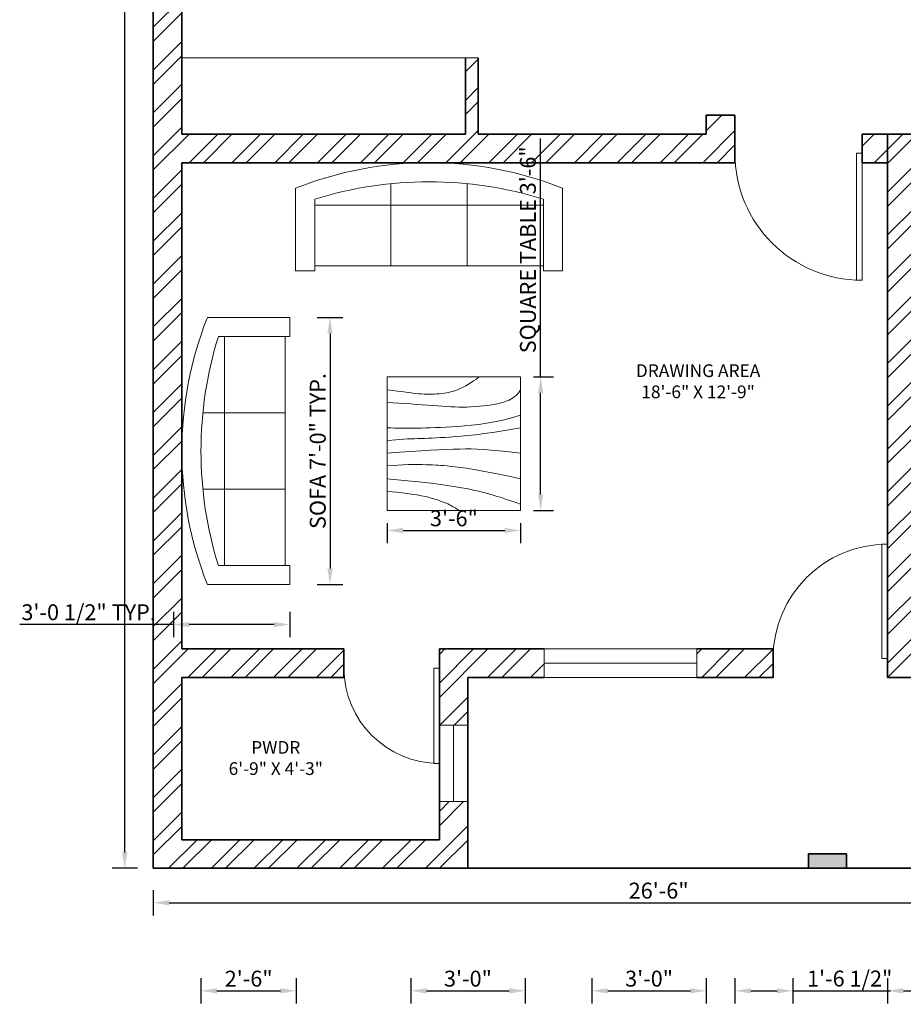
# Model space of a CAD drawing. Units: inches. Extents: x 468 to 1096, y 138 to 946.
# Tile 1 of 6: x 471 to 749, y 138 to 448. Entities that reach past the tile are written whole.
import ezdxf

# ---------------------------------------------------------------- set-up
doc = ezdxf.new("R2010")
doc.units = ezdxf.units.IN
for name, color, linetype, lineweight in [('A-ANNO-DIMS', 2, 'Continuous', 18), ('A-AREA-IDEN', 7, 'Continuous', 18), ('A-DOOR', 3, 'Continuous', 18), ('A-FLOR-CASE', 9, 'Continuous', 18), ('A-FURN', 8, 'Continuous', 18), ('A-GLAZ', 4, 'Continuous', 18), ('A-SITE-GATE', 7, 'Continuous', 35), ('A-SITE-PATT', 8, 'Continuous', 13), ('A-WALL', 7, 'Continuous', 35), ('A-WALL-PATT', 8, 'Continuous', 13), ('C-PROP', 7, 'Continuous', 35)]:
    doc.layers.add(name, color=color, linetype=linetype, lineweight=lineweight)
doc.styles.get("Standard").update_dxf_attribs({"font": 'arial.ttf'})
doc.dimstyles.new('ISO-25', dxfattribs={"dimtxt": 5, "dimasz": 5, "dimexe": 4, "dimexo": 4, "dimtad": 1, "dimdec": 1, "dimlunit": 3, "dimtxsty": 'Standard', "dimcen": 2.5, "dimadec": 0, "dimazin": 0, "dimtfac": 1, "dimtdec": 1, "dimtmove": 0, "dimatfit": 3, "dimfxl": 4, "dimfxlon": 1, "dimarcsym": 0})

# ---------------------------------------------------------------- blocks, each defined once
blk = doc.blocks.new('*U7')
for p, q in [((-40, 0), (-40, 6)), ((0, 0), (0, 6))]:
    blk.add_line(p, q)
blk.add_lwpolyline([(0, 0), (0, -40), (-1.75, -40), (-1.75, 0)], close=True)
blk.add_arc((0, 0), 40, 180, 270)
blk = doc.blocks.new('*U3')
for p, q in [((0, 0), (0, -6)), ((-36, 0), (-36, -6))]:
    blk.add_line(p, q)
blk.add_lwpolyline([(0, 0), (0, 36), (-1.75, 36), (-1.75, 0)], close=True)
blk.add_arc((0, 0), 36, 90, 180)
blk = doc.blocks.new('*U8')
for p, q in [((-30, 0), (-30, 6)), ((0, 0), (0, 6))]:
    blk.add_line(p, q)
blk.add_lwpolyline([(0, 0), (0, -30), (-1.75, -30), (-1.75, 0)], close=True)
blk.add_arc((0, 0), 30, 180, 270)
blk = doc.blocks.new('Table - Square Woodgrain 42 x 42 in.')
blk.add_line((0, -42), (42, -42))
for points in [[(0, -4), (1.704, -4.2172), (3.2358, -4.4188), (4.615, -4.604), (5.8615, -4.7721), (6.9951, -4.9224), (8.0357, -5.0541), (9.0031, -5.1667), (9.9171, -5.2594), (10.7951, -5.3316), (11.6445, -5.3836), (12.4702, -5.4157), (13.277, -5.4283), (14.0698, -5.4217), (14.8535, -5.3964), (15.6331, -5.3526), (16.4133, -5.2908), (17.1986, -5.2103), (17.9913, -5.1062), (18.793, -4.9727), (19.6056, -4.8038), (20.4307, -4.5937), (21.2701, -4.3365), (22.1256, -4.0262), (22.9989, -3.6571), (23.888, -3.2272), (24.7756, -2.7516), (25.6408, -2.2491), (26.4624, -1.7387), (27.2195, -1.2395), (27.891, -0.7703), (28.456, -0.3501), (28.8934, 0.002)], [(0, -42), (0, 0), (42, 0), (42, -42)], [(0, -8), (1.8203, -8.1001), (3.6741, -8.2149), (5.5411, -8.3408), (7.4011, -8.4741), (9.2339, -8.6112), (11.0193, -8.7484), (12.7371, -8.8821), (14.3671, -9.0086), (15.8954, -9.1246), (17.3337, -9.2278), (18.6997, -9.3159), (20.0116, -9.387), (21.2871, -9.4389), (22.5442, -9.4696), (23.8008, -9.477), (25.0749, -9.459), (26.3791, -9.4137), (27.7049, -9.3403), (29.0383, -9.2382), (30.3655, -9.1068), (31.6728, -8.9455), (32.9461, -8.7535), (34.1717, -8.5304), (35.3358, -8.2756), (36.4268, -7.9863), (37.443, -7.6521), (38.3849, -7.2603), (39.253, -6.7986), (40.048, -6.2542), (40.7705, -5.6147), (41.421, -4.8674), (42, -4)], [(42, -12), (39.1784, -12.8621), (36.4519, -13.5654), (33.8246, -14.1294), (31.3004, -14.5731), (28.8832, -14.9161), (26.577, -15.1775), (24.3858, -15.3768), (22.3136, -15.5332), (20.3622, -15.6632), (18.5254, -15.7718), (16.7947, -15.8612), (15.1618, -15.9338), (13.6183, -15.9916), (12.1558, -16.0369), (10.7659, -16.0718), (9.4403, -16.0987), (8.1703, -16.1191), (6.9461, -16.1325), (5.7577, -16.1377), (4.595, -16.1335), (3.4479, -16.1188), (2.3064, -16.0924), (1.1604, -16.0532), (0, -16)], [(42, -16), (37.6529, -16.7365), (33.8802, -17.329), (30.6179, -17.7961), (27.8015, -18.1561), (25.3668, -18.4275), (23.2497, -18.6288), (21.3859, -18.7785), (19.7111, -18.8949), (18.1693, -18.9939), (16.7375, -19.0795), (15.401, -19.1534), (14.1449, -19.217), (12.9544, -19.2717), (11.8148, -19.3191), (10.7113, -19.3606), (9.6291, -19.3976), (8.5534, -19.4323), (7.47, -19.4689), (6.3643, -19.5122), (5.222, -19.5672), (4.0288, -19.6386), (2.7703, -19.7313), (1.4321, -19.8501), (0, -20)], [(0, -24), (3.9243, -23.6805), (7.4766, -23.4138), (10.6891, -23.1954), (13.5943, -23.0205), (16.2247, -22.8847), (18.6125, -22.7832), (20.7903, -22.7116), (22.7903, -22.6651), (24.6563, -22.642), (26.4764, -22.6507), (28.35, -22.7024), (30.3766, -22.8084), (32.6555, -22.98), (35.2861, -23.2283), (38.3678, -23.5645), (42, -24)], [(42, -32), (37.392, -31.017), (33.4585, -30.2231), (30.1291, -29.5949), (27.3334, -29.109), (25.0009, -28.742), (23.0612, -28.4707), (21.4439, -28.2716), (20.0786, -28.1215), (18.8998, -28.0002), (17.8609, -27.9014), (16.9206, -27.8219), (16.0371, -27.7588), (15.1691, -27.709), (14.2748, -27.6693), (13.3128, -27.6368), (12.2415, -27.6083), (11.0295, -27.5824), (9.6867, -27.5643), (8.233, -27.5608), (6.6884, -27.5787), (5.0728, -27.6248), (3.4062, -27.7058), (1.7086, -27.8286), (0, -28)], [(0, -32), (5.4026, -32.5358), (9.9494, -33.019), (13.7424, -33.4553), (16.8834, -33.8505), (19.4743, -34.2106), (21.6171, -34.5413), (23.4136, -34.8486), (24.9657, -35.1382), (26.3614, -35.4156), (27.6332, -35.6841), (28.7995, -35.9467), (29.8788, -36.2064), (30.8897, -36.4661), (31.8507, -36.7288), (32.7802, -36.9973), (33.6968, -37.2747), (34.6175, -37.5635), (35.5531, -37.8651), (36.5128, -38.1805), (37.506, -38.5108), (38.5421, -38.8568), (39.6302, -39.2197), (40.7797, -39.6004), (42, -40)], [(0, -36), (3.0098, -36.2857), (5.5354, -36.5643), (7.6368, -36.8359), (9.374, -37.1009), (10.807, -37.3597), (11.9957, -37.6126), (13.0002, -37.8599), (13.8804, -38.102), (14.6874, -38.3393), (15.4365, -38.5729), (16.1338, -38.8041), (16.7858, -39.0341), (17.3987, -39.264), (17.9787, -39.4952), (18.5322, -39.7288), (19.0655, -39.9662), (19.5832, -40.2081), (20.0842, -40.4544), (20.5657, -40.7046), (21.0249, -40.9581), (21.459, -41.2144), (21.8653, -41.4731), (22.2409, -41.7335), (22.5831, -41.9951)]]:
    blk.add_lwpolyline(points)
blk = doc.blocks.new('Sofa - Roundback 7 ft.')
for p, q in [((-12.00002, -32.4421), (-12.00003, -6.5971)), ((11.99997, -32.4421), (11.99998, -6.5971)), ((-36.000027, -34), (-36.000027, -11.4696)), ((35.99998, -34), (35.99998, -11.4696)), ((-35.999844, -13.3819), (35.9998, -13.3819)), ((-36.000027, -32.4421), (35.99998, -32.4421))]:
    blk.add_line(p, q)
for points in [[(-36.000027, -34), (-42.000027, -34), (-42.000027, -8)], [(41.99998, -8), (41.99998, -34), (35.99998, -34)]]:
    blk.add_lwpolyline(points)
for centre, radius, start, end in [((0, -114.25), 114.25, 68.43141, 111.5686), ((-0.00001, -127.1968), 121.1968, 72.72033, 107.2797)]:
    blk.add_arc(centre, radius, start, end)
blk = doc.blocks.new('*D18')
at = {"layer": 'A-ANNO-DIMS', "color": 0, "lineweight": -2, "transparency": 16777216}
for p, q in [((508.14, 901.16), (500.14, 901.16)), ((504.14, 186.16), (504.14, 896.16)), ((508.14, 181.16), (500.14, 181.16))]:
    blk.add_line(p, q, dxfattribs=at)
at = {"layer": 'A-ANNO-DIMS', "color": 0, "transparency": 16777216}
for points in [[(503.3, 896.16), (504.97, 896.16), (504.14, 901.16)], [(503.3, 186.16), (504.97, 186.16), (504.14, 181.16)]]:
    blk.add_solid(points, dxfattribs=at)
at = {"layer": 'Defpoints', "color": 0, "transparency": 16777216}
for p in [(504.14, 901.16), (513.13, 901.16), (513.13, 181.16)]:
    blk.add_point(p, dxfattribs=at)
at = {"layer": 'A-ANNO-DIMS', "color": 0, "transparency": 16777216, "insert": (500.96, 541.16), "char_height": 5, "attachment_point": 5, "rotation": 90}
blk.add_mtext("60'", dxfattribs=at)
blk = doc.blocks.new('*D19')
at = {"layer": 'A-ANNO-DIMS', "color": 0, "lineweight": -2, "transparency": 16777216}
for p, q in [((513.13, 174.32), (513.13, 166.32)), ((831.13, 174.32), (831.13, 166.32)), ((518.13, 170.32), (826.13, 170.32))]:
    blk.add_line(p, q, dxfattribs=at)
at = {"layer": 'A-ANNO-DIMS', "color": 0, "transparency": 16777216}
for points in [[(518.13, 171.15), (518.13, 169.48), (513.13, 170.32)], [(826.13, 171.15), (826.13, 169.48), (831.13, 170.32)]]:
    blk.add_solid(points, dxfattribs=at)
at = {"layer": 'Defpoints', "color": 0, "transparency": 16777216}
for p in [(513.13, 181.16), (831.13, 181.16), (831.13, 170.32)]:
    blk.add_point(p, dxfattribs=at)
at = {"layer": 'A-ANNO-DIMS', "color": 0, "transparency": 16777216, "insert": (672.13, 173.49), "char_height": 5, "attachment_point": 5}
blk.add_mtext('26\'-6"', dxfattribs=at)
blk = doc.blocks.new('WIN-24-W9')
for p, q in [((0, 24), (9, 24)), ((4.5, 24), (4.5, 0)), ((0, 0), (9, 0))]:
    blk.add_line(p, q)
blk = doc.blocks.new('WIN-48-W9')
for p, q in [((0, 0), (0, 9)), ((48, 0), (48, 9)), ((0, 4.5), (48, 4.5))]:
    blk.add_line(p, q)
blk = doc.blocks.new('*D37')
at = {"layer": 'A-ANNO-DIMS', "color": 0, "lineweight": -2, "transparency": 16777216}
for p, q in [((564.73, 354.45), (572.73, 354.45)), ((568.73, 349.45), (568.73, 275.45)), ((564.73, 270.45), (572.73, 270.45))]:
    blk.add_line(p, q, dxfattribs=at)
at = {"layer": 'A-ANNO-DIMS', "color": 0, "transparency": 16777216}
for points in [[(567.9, 349.45), (569.56, 349.45), (568.73, 354.45)], [(567.9, 275.45), (569.56, 275.45), (568.73, 270.45)]]:
    blk.add_solid(points, dxfattribs=at)
at = {"layer": 'Defpoints', "color": 0, "transparency": 16777216}
for p in [(556.13, 354.45), (556.13, 270.45), (568.73, 270.45)]:
    blk.add_point(p, dxfattribs=at)
at = {"layer": 'A-ANNO-DIMS', "color": 0, "transparency": 16777216, "insert": (565.52, 312.45), "char_height": 5, "attachment_point": 5, "rotation": 90}
blk.add_mtext('SOFA 7\'-0" TYP.', dxfattribs=at)
blk = doc.blocks.new('*D38')
at = {"layer": 'A-ANNO-DIMS', "color": 0, "lineweight": -2, "transparency": 16777216}
for p, q in [((519.46, 261.85), (519.46, 253.85)), ((556.13, 261.85), (556.13, 253.85)), ((519.46, 257.85), (471.09, 257.85)), ((551.13, 257.85), (524.46, 257.85))]:
    blk.add_line(p, q, dxfattribs=at)
at = {"layer": 'A-ANNO-DIMS', "color": 0, "transparency": 16777216}
for points in [[(524.46, 258.69), (524.46, 257.02), (519.46, 257.85)], [(551.13, 258.69), (551.13, 257.02), (556.13, 257.85)]]:
    blk.add_solid(points, dxfattribs=at)
at = {"layer": 'Defpoints', "color": 0, "transparency": 16777216}
for p in [(519.46, 270.45), (556.13, 270.45), (519.46, 257.85)]:
    blk.add_point(p, dxfattribs=at)
at = {"layer": 'A-ANNO-DIMS', "color": 0, "transparency": 16777216, "insert": (492.78, 261.07), "char_height": 5, "attachment_point": 5}
blk.add_mtext('3\'-0 1/2" TYP.', dxfattribs=at)
blk = doc.blocks.new('*D53')
at = {"layer": 'A-ANNO-DIMS', "color": 0, "lineweight": -2, "transparency": 16777216}
for p, q in [((635.01, 335.75), (635.01, 410.78)), ((632.71, 335.75), (639.01, 335.75)), ((635.01, 298.75), (635.01, 330.75)), ((632.71, 293.75), (639.01, 293.75))]:
    blk.add_line(p, q, dxfattribs=at)
at = {"layer": 'A-ANNO-DIMS', "color": 0, "transparency": 16777216}
for points in [[(634.18, 330.75), (635.84, 330.75), (635.01, 335.75)], [(634.18, 298.75), (635.84, 298.75), (635.01, 293.75)]]:
    blk.add_solid(points, dxfattribs=at)
at = {"layer": 'Defpoints', "color": 0, "transparency": 16777216}
for p in [(628.71, 335.75), (635.01, 335.75), (628.71, 293.75)]:
    blk.add_point(p, dxfattribs=at)
at = {"layer": 'A-ANNO-DIMS', "color": 0, "transparency": 16777216, "insert": (631.65, 375.76), "char_height": 5, "attachment_point": 5, "rotation": 90}
blk.add_mtext('SQUARE TABLE 3\'-6"', dxfattribs=at)
blk = doc.blocks.new('*D54')
at = {"layer": 'A-ANNO-DIMS', "color": 0, "lineweight": -2, "transparency": 16777216}
for p, q in [((586.71, 289.75), (586.71, 283.45)), ((628.71, 289.75), (628.71, 283.45)), ((591.71, 287.45), (623.71, 287.45))]:
    blk.add_line(p, q, dxfattribs=at)
at = {"layer": 'A-ANNO-DIMS', "color": 0, "transparency": 16777216}
for points in [[(591.71, 288.28), (591.71, 286.62), (586.71, 287.45)], [(623.71, 288.28), (623.71, 286.62), (628.71, 287.45)]]:
    blk.add_solid(points, dxfattribs=at)
at = {"layer": 'Defpoints', "color": 0, "transparency": 16777216}
for p in [(586.71, 293.75), (628.71, 293.75), (628.71, 287.45)]:
    blk.add_point(p, dxfattribs=at)
at = {"layer": 'A-ANNO-DIMS', "color": 0, "transparency": 16777216, "insert": (607.71, 290.63), "char_height": 5, "attachment_point": 5}
blk.add_mtext('3\'-6"', dxfattribs=at)
blk = doc.blocks.new('*D55')
at = {"layer": 'A-ANNO-DIMS', "color": 0, "lineweight": -2, "transparency": 16777216}
for p, q in [((744.13, 146.61), (744.13, 138.61)), ((858.13, 146.61), (858.13, 138.61)), ((749.13, 142.61), (853.13, 142.61))]:
    blk.add_line(p, q, dxfattribs=at)
at = {"layer": 'A-ANNO-DIMS', "color": 0, "transparency": 16777216}
for points in [[(749.13, 143.44), (749.13, 141.78), (744.13, 142.61)], [(853.13, 143.44), (853.13, 141.78), (858.13, 142.61)]]:
    blk.add_solid(points, dxfattribs=at)
at = {"layer": 'Defpoints', "color": 0, "transparency": 16777216}
for p in [(744.13, 241.16), (858.13, 241.16), (858.13, 142.61)]:
    blk.add_point(p, dxfattribs=at)
at = {"layer": 'A-ANNO-DIMS', "color": 0, "transparency": 16777216, "insert": (801.13, 145.79), "char_height": 5, "attachment_point": 5}
blk.add_mtext('9\'-6"', dxfattribs=at)
blk = doc.blocks.new('*D61')
at = {"layer": 'A-ANNO-DIMS', "color": 0, "lineweight": -2, "transparency": 16777216}
for p, q in [((594.13, 146.61), (594.13, 138.61)), ((630.13, 146.61), (630.13, 138.61)), ((599.13, 142.61), (625.13, 142.61))]:
    blk.add_line(p, q, dxfattribs=at)
at = {"layer": 'A-ANNO-DIMS', "color": 0, "transparency": 16777216}
for points in [[(599.13, 143.44), (599.13, 141.78), (594.13, 142.61)], [(625.13, 143.44), (625.13, 141.78), (630.13, 142.61)]]:
    blk.add_solid(points, dxfattribs=at)
at = {"layer": 'Defpoints', "color": 0, "transparency": 16777216}
for p in [(594.13, 829.16), (630.13, 826.16), (630.13, 142.61)]:
    blk.add_point(p, dxfattribs=at)
at = {"layer": 'A-ANNO-DIMS', "color": 0, "transparency": 16777216, "insert": (612.13, 145.79), "char_height": 5, "attachment_point": 5}
blk.add_mtext('3\'-0"', dxfattribs=at)
blk = doc.blocks.new('*D66')
at = {"layer": 'A-ANNO-DIMS', "color": 0, "lineweight": -2, "transparency": 16777216}
for p, q in [((696.13, 146.61), (696.13, 138.61)), ((714.39, 146.61), (714.39, 138.61)), ((701.13, 142.61), (709.39, 142.61)), ((714.39, 142.61), (745.11, 142.61))]:
    blk.add_line(p, q, dxfattribs=at)
at = {"layer": 'A-ANNO-DIMS', "color": 0, "transparency": 16777216}
for points in [[(701.13, 143.44), (701.13, 141.78), (696.13, 142.61)], [(709.39, 143.44), (709.39, 141.78), (714.39, 142.61)]]:
    blk.add_solid(points, dxfattribs=at)
at = {"layer": 'Defpoints', "color": 0, "transparency": 16777216}
for p in [(696.13, 820.16), (714.39, 802.16), (714.39, 142.61)]:
    blk.add_point(p, dxfattribs=at)
at = {"layer": 'A-ANNO-DIMS', "color": 0, "transparency": 16777216, "insert": (732.25, 145.82), "char_height": 5, "attachment_point": 5}
blk.add_mtext('1\'-6 1/2"', dxfattribs=at)
blk = doc.blocks.new('*D75')
at = {"layer": 'A-ANNO-DIMS', "color": 0, "lineweight": -2, "transparency": 16777216}
for p, q in [((696.13, 935.71), (696.13, 943.71)), ((736.13, 935.71), (736.13, 943.71)), ((701.13, 939.71), (731.13, 939.71))]:
    blk.add_line(p, q, dxfattribs=at)
at = {"layer": 'A-ANNO-DIMS', "color": 0, "transparency": 16777216}
for points in [[(701.13, 940.54), (701.13, 938.88), (696.13, 939.71)], [(731.13, 940.54), (731.13, 938.88), (736.13, 939.71)]]:
    blk.add_solid(points, dxfattribs=at)
at = {"layer": 'Defpoints', "color": 0, "transparency": 16777216}
for p in [(736.13, 939.71), (696.13, 412.16), (736.13, 412.16)]:
    blk.add_point(p, dxfattribs=at)
at = {"layer": 'A-ANNO-DIMS', "color": 0, "transparency": 16777216, "insert": (716.13, 942.89), "char_height": 5, "attachment_point": 5}
blk.add_mtext('3\'-4"', dxfattribs=at)
blk = doc.blocks.new('*D76')
at = {"layer": 'A-ANNO-DIMS', "color": 0, "lineweight": -2, "transparency": 16777216}
for p, q in [((1087.68, 454.16), (1095.68, 454.16)), ((1091.68, 423.16), (1091.68, 449.16)), ((1087.68, 418.16), (1095.68, 418.16))]:
    blk.add_line(p, q, dxfattribs=at)
at = {"layer": 'A-ANNO-DIMS', "color": 0, "transparency": 16777216}
for points in [[(1090.85, 449.16), (1092.51, 449.16), (1091.68, 454.16)], [(1090.85, 423.16), (1092.51, 423.16), (1091.68, 418.16)]]:
    blk.add_solid(points, dxfattribs=at)
at = {"layer": 'Defpoints', "color": 0, "transparency": 16777216}
for p in [(687.13, 454.16), (1091.68, 454.16), (687.13, 418.16)]:
    blk.add_point(p, dxfattribs=at)
at = {"layer": 'A-ANNO-DIMS', "color": 0, "transparency": 16777216, "insert": (1088.5, 436.16), "char_height": 5, "attachment_point": 5, "rotation": 90}
blk.add_mtext('3\'-0"', dxfattribs=at)
blk = doc.blocks.new('*D77')
at = {"layer": 'A-ANNO-DIMS', "color": 0, "lineweight": -2, "transparency": 16777216}
for p, q in [((651.13, 146.61), (651.13, 138.61)), ((687.13, 146.61), (687.13, 138.61)), ((656.13, 142.61), (682.13, 142.61))]:
    blk.add_line(p, q, dxfattribs=at)
at = {"layer": 'A-ANNO-DIMS', "color": 0, "transparency": 16777216}
for points in [[(656.13, 143.44), (656.13, 141.78), (651.13, 142.61)], [(682.13, 143.44), (682.13, 141.78), (687.13, 142.61)]]:
    blk.add_solid(points, dxfattribs=at)
at = {"layer": 'Defpoints', "color": 0, "transparency": 16777216}
for p in [(651.13, 565.16), (687.13, 565.16), (687.13, 142.61)]:
    blk.add_point(p, dxfattribs=at)
at = {"layer": 'A-ANNO-DIMS', "color": 0, "transparency": 16777216, "insert": (669.13, 145.79), "char_height": 5, "attachment_point": 5}
blk.add_mtext('3\'-0"', dxfattribs=at)
blk = doc.blocks.new('*D78')
at = {"layer": 'A-ANNO-DIMS', "color": 0, "lineweight": -2, "transparency": 16777216}
for p, q in [((573.13, 935.71), (573.13, 943.71)), ((603.13, 935.71), (603.13, 943.71)), ((578.13, 939.71), (598.13, 939.71))]:
    blk.add_line(p, q, dxfattribs=at)
at = {"layer": 'A-ANNO-DIMS', "color": 0, "transparency": 16777216}
for points in [[(578.13, 940.54), (578.13, 938.88), (573.13, 939.71)], [(598.13, 940.54), (598.13, 938.88), (603.13, 939.71)]]:
    blk.add_solid(points, dxfattribs=at)
at = {"layer": 'Defpoints', "color": 0, "transparency": 16777216}
for p in [(603.13, 939.71), (573.13, 250.16), (603.13, 250.16)]:
    blk.add_point(p, dxfattribs=at)
at = {"layer": 'A-ANNO-DIMS', "color": 0, "transparency": 16777216, "insert": (588.13, 942.89), "char_height": 5, "attachment_point": 5}
blk.add_mtext('2\'-6"', dxfattribs=at)
blk = doc.blocks.new('*D79')
at = {"layer": 'A-ANNO-DIMS', "color": 0, "lineweight": -2, "transparency": 16777216}
for p, q in [((612.13, 935.71), (612.13, 943.71)), ((636.13, 935.71), (636.13, 943.71)), ((617.13, 939.71), (631.13, 939.71))]:
    blk.add_line(p, q, dxfattribs=at)
at = {"layer": 'A-ANNO-DIMS', "color": 0, "transparency": 16777216}
for points in [[(617.13, 940.54), (617.13, 938.88), (612.13, 939.71)], [(631.13, 940.54), (631.13, 938.88), (636.13, 939.71)]]:
    blk.add_solid(points, dxfattribs=at)
at = {"layer": 'Defpoints', "color": 0, "transparency": 16777216}
for p in [(636.13, 939.71), (612.13, 241.16), (636.13, 241.16)]:
    blk.add_point(p, dxfattribs=at)
at = {"layer": 'A-ANNO-DIMS', "color": 0, "transparency": 16777216, "insert": (624.13, 942.89), "char_height": 5, "attachment_point": 5}
blk.add_mtext('2\'-0"', dxfattribs=at)
blk = doc.blocks.new('*D80')
at = {"layer": 'A-ANNO-DIMS', "color": 0, "lineweight": -2, "transparency": 16777216}
for p, q in [((684.13, 935.71), (684.13, 943.71)), ((708.13, 935.71), (708.13, 943.71)), ((689.13, 939.71), (703.13, 939.71))]:
    blk.add_line(p, q, dxfattribs=at)
at = {"layer": 'A-ANNO-DIMS', "color": 0, "transparency": 16777216}
for points in [[(689.13, 940.54), (689.13, 938.88), (684.13, 939.71)], [(703.13, 940.54), (703.13, 938.88), (708.13, 939.71)]]:
    blk.add_solid(points, dxfattribs=at)
at = {"layer": 'Defpoints', "color": 0, "transparency": 16777216}
for p in [(708.13, 939.71), (684.13, 250.16), (708.13, 250.16)]:
    blk.add_point(p, dxfattribs=at)
at = {"layer": 'A-ANNO-DIMS', "color": 0, "transparency": 16777216, "insert": (696.13, 942.89), "char_height": 5, "attachment_point": 5}
blk.add_mtext('2\'-0"', dxfattribs=at)
blk = doc.blocks.new('*D81')
at = {"layer": 'A-ANNO-DIMS', "color": 0, "lineweight": -2, "transparency": 16777216}
for p, q in [((708.13, 935.71), (708.13, 943.71)), ((744.13, 935.71), (744.13, 943.71)), ((713.13, 939.71), (739.13, 939.71))]:
    blk.add_line(p, q, dxfattribs=at)
at = {"layer": 'A-ANNO-DIMS', "color": 0, "transparency": 16777216}
for points in [[(713.13, 940.54), (713.13, 938.88), (708.13, 939.71)], [(739.13, 940.54), (739.13, 938.88), (744.13, 939.71)]]:
    blk.add_solid(points, dxfattribs=at)
at = {"layer": 'Defpoints', "color": 0, "transparency": 16777216}
for p in [(744.13, 939.71), (708.13, 250.16), (744.13, 250.16)]:
    blk.add_point(p, dxfattribs=at)
at = {"layer": 'A-ANNO-DIMS', "color": 0, "transparency": 16777216, "insert": (726.13, 942.89), "char_height": 5, "attachment_point": 5}
blk.add_mtext('3\'-0"', dxfattribs=at)
blk = doc.blocks.new('*D85')
at = {"layer": 'A-ANNO-DIMS', "color": 0, "lineweight": -2, "transparency": 16777216}
for p, q in [((528.13, 146.61), (528.13, 138.61)), ((558.13, 146.61), (558.13, 138.61)), ((533.13, 142.61), (553.13, 142.61))]:
    blk.add_line(p, q, dxfattribs=at)
at = {"layer": 'A-ANNO-DIMS', "color": 0, "transparency": 16777216}
for points in [[(533.13, 143.44), (533.13, 141.78), (528.13, 142.61)], [(553.13, 143.44), (553.13, 141.78), (558.13, 142.61)]]:
    blk.add_solid(points, dxfattribs=at)
at = {"layer": 'Defpoints', "color": 0, "transparency": 16777216}
for p in [(528.13, 565.16), (558.13, 565.16), (558.13, 142.61)]:
    blk.add_point(p, dxfattribs=at)
at = {"layer": 'A-ANNO-DIMS', "color": 0, "transparency": 16777216, "insert": (543.13, 145.79), "char_height": 5, "attachment_point": 5}
blk.add_mtext('2\'-6"', dxfattribs=at)

msp = doc.modelspace()

# ---------------------------------------------------------------- hatches: boundary and pattern name
at = {"layer": 'A-SITE-PATT'}
h = msp.add_hatch(color=256, dxfattribs=at)
h.dxf.hatch_style = 1
h.paths.add_polyline_path([(731.29, 185.66), (719.29, 185.66), (719.29, 181.16), (731.29, 181.16)])
h.paths.add_polyline_path([(843.13, 190.16), (831.13, 190.16), (831.13, 181.16), (843.13, 181.16)])
h.paths.add_polyline_path([(897.13, 190.16), (885.13, 190.16), (885.13, 181.16), (897.13, 181.16)])
h.paths.add_polyline_path([(1053.13, 190.16), (1041.13, 190.16), (1041.13, 181.16), (1053.13, 181.16)])
at = {"layer": 'A-WALL-PATT'}
h = msp.add_hatch(dxfattribs=at)
h.set_pattern_fill('ANSI32', color=256)
h.paths.add_polyline_path([(639.13, 901.16), (513.13, 901.16), (513.13, 181.16), (612.13, 181.16), (612.13, 202.16), (603.13, 202.16), (603.13, 190.16), (522.13, 190.16), (522.13, 241.16), (573.13, 241.16), (573.13, 250.16), (522.13, 250.16), (522.13, 403.16), (696.13, 403.16), (696.13, 418.16), (687.13, 418.16), (687.13, 412.16), (615.37, 412.16), (615.37, 436.16), (611.37, 436.16), (611.37, 412.16), (522.13, 412.16), (522.13, 436.16), (522.13, 565.16), (528.13, 565.16), (528.13, 571.16), (522.13, 571.16), (522.13, 625.16), (531.13, 625.16), (531.13, 634.16), (522.13, 634.16), (522.13, 820.16), (590.13, 820.16), (590.13, 796.16), (594.13, 796.16), (594.13, 820.16), (594.13, 826.16), (594.13, 829.16), (522.13, 829.16), (522.13, 892.16), (630.13, 892.16), (630.13, 872.66), (639.13, 872.66)])
h = msp.add_hatch(dxfattribs=at)
h.set_pattern_fill('ANSI32', color=256)
h.paths.add_polyline_path([(1053.13, 412.16), (1044.13, 412.16), (1044.13, 241.16), (1053.13, 241.16)])
h.paths.add_polyline_path([(996.13, 448.16), (987.13, 448.16), (987.13, 412.16), (942.13, 412.16), (942.13, 403.16), (996.13, 403.16)])
h.paths.add_polyline_path([(996.13, 532.16), (987.13, 532.16), (987.13, 496.16), (996.13, 496.16)])
h.paths.add_polyline_path([(996.13, 646.16), (987.13, 646.16), (987.13, 607.16), (813.13, 607.16), (813.13, 598.16), (822.13, 598.16), (987.13, 598.16), (987.13, 592.16), (996.13, 592.16), (996.13, 598.16), (996.13, 607.16)])
h.paths.add_polyline_path([(894.13, 412.16), (849.13, 412.16), (849.13, 403.16), (894.13, 403.16)])
h.paths.add_polyline_path([(801.13, 412.16), (744.13, 412.16), (744.13, 250.16), (744.13, 241.16), (777.13, 241.16), (777.13, 250.16), (753.13, 250.16), (753.13, 403.16), (801.13, 403.16)])
h.paths.add_polyline_path([(744.13, 412.16), (736.13, 412.16), (736.13, 403.16), (744.13, 403.16)])
h = msp.add_hatch(dxfattribs=at)
h.set_pattern_fill('ANSI32', color=256)
h.paths.add_polyline_path([(636.13, 250.16), (603.13, 250.16), (603.13, 244.16), (603.13, 226.16), (612.13, 226.16), (612.13, 241.16), (636.13, 241.16)])
h.paths.add_polyline_path([(708.13, 247.16), (708.13, 250.16), (684.13, 250.16), (684.13, 241.16), (708.13, 241.16)])

# ---------------------------------------------------------------- linework, layer by layer
at = {"layer": 'A-FLOR-CASE'}
for p, q in [((522.13, 412.16), (522.13, 436.16)), ((522.13, 436.16), (615.37, 436.16))]:
    msp.add_line(p, q, dxfattribs=at)
at = {"layer": 'A-GLAZ'}
for p, q in [((636.13, 250.16), (684.13, 250.16)), ((636.13, 241.16), (684.13, 241.16))]:
    msp.add_line(p, q, dxfattribs=at)
at = {"layer": 'A-SITE-GATE'}
for p, q in [((731.29, 185.66), (719.29, 185.66)), ((719.29, 185.66), (719.29, 181.16)), ((731.29, 181.16), (731.29, 185.66))]:
    msp.add_line(p, q, dxfattribs=at)
at = {"layer": 'A-WALL'}
for p, q in [((522.13, 565.16), (522.13, 412.16)), ((611.37, 436.16), (611.37, 412.16)), ((615.37, 436.16), (615.37, 412.16)), ((687.13, 412.16), (687.13, 418.16)), ((687.13, 418.16), (696.13, 418.16)), ((696.13, 418.16), (696.13, 403.16)), ((611.37, 412.16), (522.13, 412.16)), ((687.13, 412.16), (615.37, 412.16)), ((744.13, 412.16), (736.13, 412.16)), ((736.13, 412.16), (736.13, 403.16)), ((744.13, 412.16), (801.13, 412.16)), ((744.13, 412.16), (744.13, 250.16)), ((696.13, 403.16), (522.13, 403.16)), ((522.13, 403.16), (522.13, 250.16)), ((736.13, 403.16), (744.13, 403.16)), ((573.13, 250.16), (522.13, 250.16)), ((573.13, 250.16), (573.13, 241.16)), ((603.13, 250.16), (603.13, 202.16)), ((603.13, 250.16), (636.13, 250.16)), ((708.13, 250.16), (684.13, 250.16)), ((708.13, 241.16), (708.13, 250.16)), ((744.13, 250.16), (744.13, 241.16)), ((522.13, 241.16), (522.13, 190.16)), ((522.13, 241.16), (573.13, 241.16)), ((612.13, 241.16), (612.13, 202.16)), ((612.13, 241.16), (636.13, 241.16)), ((684.13, 241.16), (708.13, 241.16)), ((744.13, 241.16), (840.13, 241.16)), ((603.13, 202.16), (603.13, 190.16)), ((612.13, 202.16), (612.13, 181.16)), ((522.13, 190.16), (603.13, 190.16))]:
    msp.add_line(p, q, dxfattribs=at)
at = {"layer": 'C-PROP'}
for p, q in [((513.13, 901.16), (513.13, 181.16)), ((513.13, 181.16), (1053.13, 181.16))]:
    msp.add_line(p, q, dxfattribs=at)

# ---------------------------------------------------------------- block references
at = {"layer": 'A-DOOR'}
for name, p in [('*U7', (736.13, 406.16)), ('*U3', (744.13, 247.16)), ('*U8', (603.13, 244.16))]:
    msp.add_blockref(name, p, dxfattribs=at)
at = {"layer": 'A-FURN', "xscale": -1}
msp.add_blockref('Sofa - Roundback 7 ft.', (599.91, 403.16), dxfattribs=at)
at = {"layer": 'A-FURN', "xscale": -1, "rotation": 90}
msp.add_blockref('Sofa - Roundback 7 ft.', (522.13, 312.45), dxfattribs=at)
at = {"layer": 'A-FURN'}
msp.add_blockref('Table - Square Woodgrain 42 x 42 in.', (586.71, 335.75), dxfattribs=at)
at = {"layer": 'A-GLAZ'}
for name, p in [('WIN-48-W9', (636.13, 241.16)), ('WIN-24-W9', (603.13, 202.16))]:
    msp.add_blockref(name, p, dxfattribs=at)

# ---------------------------------------------------------------- texts
at = {"layer": 'A-AREA-IDEN', "char_height": 4, "attachment_point": 1}
for s, width, insert in [('\\pxqc;DRAWING AREA\\P18\'-6" X 12\'-9"', 55.2509, (656.92, 339.73)), ('\\pxqc;PWDR\\P6\'-9" X 4\'-3"', 36.2598, (533.54, 221.19))]:
    msp.add_mtext_dynamic_manual_height_columns(s, width=width, gutter_width=12.5, heights=[0], dxfattribs=dict(at, insert=insert))

# ---------------------------------------------------------------- dimensions: what is measured, and where the dimension line sits
at = {"layer": 'A-ANNO-DIMS'}
for base, p1, p2, override, picture, middle in [((603.13, 939.71), (573.13, 250.16), (603.13, 250.16), {"dimdec": 1, "dimlfac": 1, "dimrnd": 0, "dimzin": 1, "dimdsep": 46, "dimlunit": 4, "dimfrac": 2}, '*D78', (588.13, 942.89)), ((636.13, 939.71), (612.13, 241.16), (636.13, 241.16), {"dimdec": 1, "dimlfac": 1, "dimrnd": 0, "dimzin": 1, "dimdsep": 46, "dimlunit": 4, "dimfrac": 2}, '*D79', (624.13, 942.89)), ((708.13, 939.71), (684.13, 250.16), (708.13, 250.16), {"dimdec": 1, "dimlfac": 1, "dimrnd": 0, "dimzin": 1, "dimdsep": 46, "dimlunit": 4, "dimfrac": 2}, '*D80', (696.13, 942.89)), ((736.13, 939.71), (696.13, 412.16), (736.13, 412.16), {"dimdec": 1, "dimlfac": 1, "dimrnd": 0, "dimzin": 1, "dimdsep": 46, "dimlunit": 4, "dimfrac": 2}, '*D75', (716.13, 942.89)), ((744.13, 939.71), (708.13, 250.16), (744.13, 250.16), {"dimdec": 1, "dimlfac": 1, "dimrnd": 0, "dimzin": 1, "dimdsep": 46, "dimlunit": 4, "dimfrac": 2}, '*D81', (726.13, 942.89)), ((630.13, 142.61), (594.13, 829.16), (630.13, 826.16), {"dimdec": 1, "dimlfac": 1, "dimrnd": 0, "dimzin": 1, "dimdsep": 46, "dimlunit": 4, "dimfrac": 2}, '*D61', (612.13, 145.79)), ((714.39, 142.61), (696.13, 820.16), (714.39, 802.16), {"dimdec": 1, "dimlfac": 1, "dimrnd": 0, "dimzin": 1, "dimdsep": 46, "dimlunit": 4, "dimfrac": 2}, '*D66', (732.25, 145.82)), ((558.13, 142.61), (528.13, 565.16), (558.13, 565.16), {"dimdec": 1, "dimlfac": 1, "dimrnd": 0, "dimzin": 1, "dimdsep": 46, "dimlunit": 4, "dimfrac": 2}, '*D85', (543.13, 145.79)), ((687.13, 142.61), (651.13, 565.16), (687.13, 565.16), {"dimdec": 1, "dimlfac": 1, "dimrnd": 0, "dimzin": 1, "dimdsep": 46, "dimlunit": 4, "dimfrac": 2}, '*D77', (669.13, 145.79)), ((628.71, 287.45), (586.71, 293.75), (628.71, 293.75), {"dimdec": 1, "dimlfac": 1, "dimrnd": 0, "dimzin": 1, "dimdsep": 46, "dimlunit": 4, "dimfrac": 2}, '*D54', (607.71, 290.63)), ((858.13, 142.61), (744.13, 241.16), (858.13, 241.16), {"dimdec": 1, "dimlfac": 1, "dimrnd": 0, "dimzin": 1, "dimdsep": 46, "dimlunit": 4, "dimfrac": 2}, '*D55', (801.13, 145.79)), ((831.13, 170.32), (513.13, 181.16), (831.13, 181.16), {"dimclrd": 0, "dimclre": 0, "dimclrt": 0}, '*D19', (672.13, 173.49))]:
    dim = msp.add_linear_dim(base=base, p1=p1, p2=p2, dimstyle='ISO-25', override=override, dxfattribs=at)
    dim.commit()
    dim.dimension.update_dxf_attribs({"geometry": picture, "text_midpoint": middle})
for base, p1, p2, override, picture, middle in [((504.14, 901.16), (513.13, 181.16), (513.13, 901.16), {"dimclrd": 0, "dimclre": 0, "dimclrt": 0}, '*D18', (500.96, 541.16)), ((1091.68, 454.16), (687.13, 418.16), (687.13, 454.16), {"dimdec": 1, "dimlfac": 1, "dimrnd": 0, "dimzin": 1, "dimdsep": 46, "dimlunit": 4, "dimfrac": 2}, '*D76', (1088.5, 436.16))]:
    dim = msp.add_linear_dim(base=base, p1=p1, p2=p2, angle=90, dimstyle='ISO-25', override=override, dxfattribs=at)
    dim.commit()
    dim.dimension.update_dxf_attribs({"geometry": picture, "text_midpoint": middle})
for base, p1, p2, angle, text, picture, middle in [((635.01, 335.75), (628.71, 293.75), (628.71, 335.75), 90, 'SQUARE TABLE <>', '*D53', (631.65, 375.76)), ((568.73, 270.45), (556.13, 354.45), (556.13, 270.45), 270, 'SOFA <> TYP.', '*D37', (565.52, 312.45)), ((519.46, 257.85), (556.13, 270.45), (519.46, 270.45), 180, '<> TYP.', '*D38', (492.78, 261.07))]:
    dim = msp.add_linear_dim(base=base, p1=p1, p2=p2, angle=angle, text=text, dimstyle='ISO-25', override={"dimdec": 1, "dimlfac": 1, "dimrnd": 0, "dimzin": 1, "dimdsep": 46, "dimlunit": 4, "dimfrac": 2}, dxfattribs=at)
    dim.commit()
    dim.dimension.update_dxf_attribs({"geometry": picture, "text_midpoint": middle})

doc.saveas('drawing.dxf')
